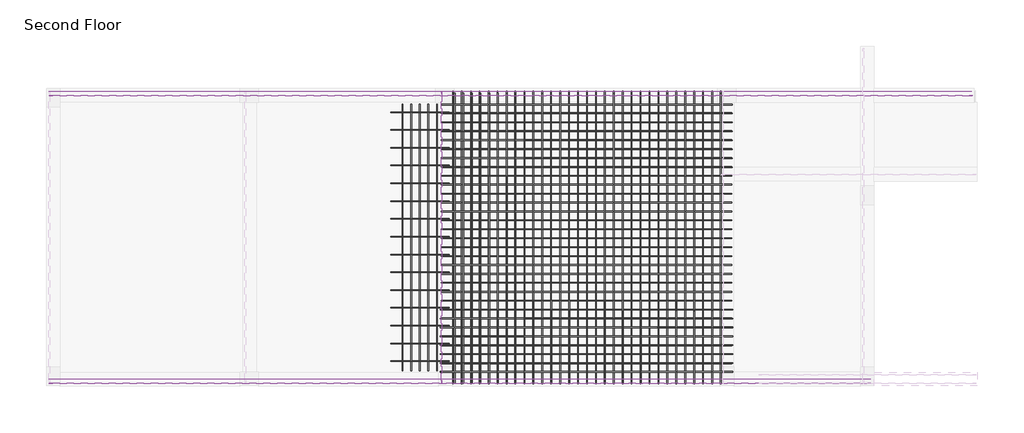
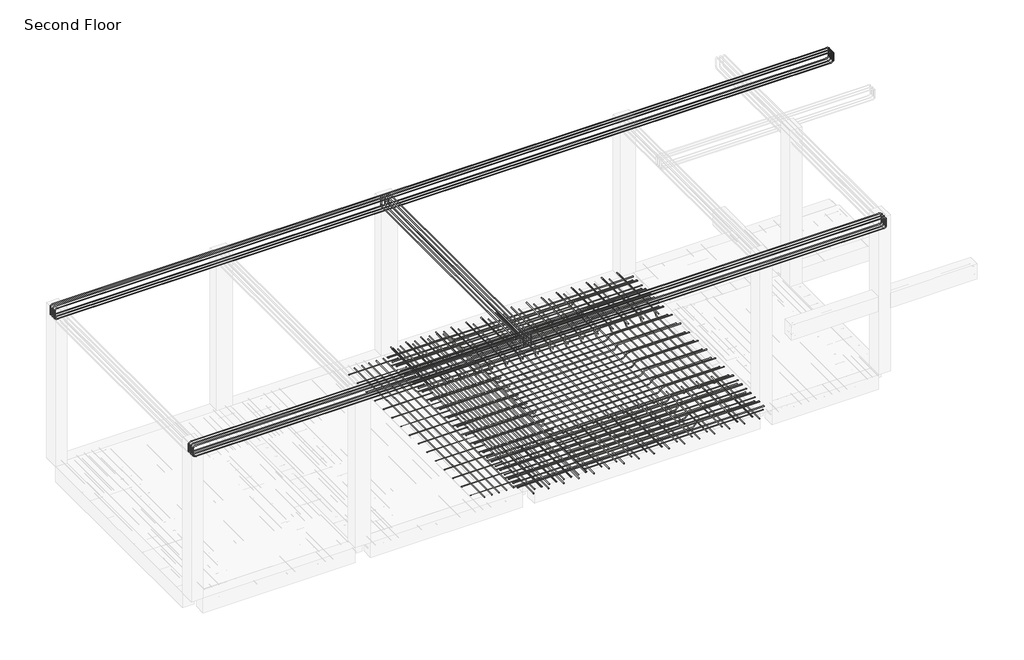
# One storey, part 3 of 4: 18 reinforcing bars.
"""IFC4 building model written with IfcOpenShell, lengths in millimetres."""

from ifc_helpers import new_model, si_unit, point, frame, origin, place, context, project, spatial, polyline, circle_curve, trimmed, segment, composite_curve, source, transform, mapped, element, save
from ifc_brep_helpers import swept_disk

model = new_model("IFC4")

# Units and contexts
model_context = context("Model", 3, world=origin())
ifc_project = project(units=[si_unit("LENGTHUNIT", "METRE", prefix="MILLI")], contexts=[model_context])

# Site, building, storey
site = spatial("IfcSite", under=ifc_project)
building = spatial("IfcBuilding", under=site)
storey = spatial("IfcBuildingStorey", under=building, Name="Second Floor", Elevation=6400.8)

# Reinforcing bars
placement = place(None, origin())
reinforcing_bar_shape = source(origin(), model_context, "Body", "SolidModel", [
    swept_disk(composite_curve([segment(polyline([(-2909.6112474, 5017.2334631, 9364.0994949), (-2909.6112474, 5017.2334631, 9512.0994949)]), True, "CONTINUOUS"), segment(trimmed(circle_curve(frame((-2909.6112474, 4971.2334631, 9512.0994949), z_axis=(1.0, 0.0, 0.0), x_axis=(0.0, 46.0, 0.0)), 46.0), [point((-2909.6112474, 5017.2334631, 9512.0994949))], [point((-2909.6112474, 4971.2334631, 9558.0994949))], True, "CARTESIAN"), True, "CONTINUOUS"), segment(polyline([(-2909.6112474, 4971.2334631, 9558.0994949), (-2909.6112474, 278.4334631, 9558.0994949)]), True, "CONTINUOUS"), segment(trimmed(circle_curve(frame((-2909.6112474, 278.4334631, 9512.0994949), z_axis=(1.0, 0.0, 0.0), x_axis=(0.0, 0.0, 46.0)), 46.0), [point((-2909.6112474, 278.4334631, 9558.0994949))], [point((-2909.6112474, 232.4334631, 9512.0994949))], True, "CARTESIAN"), True, "CONTINUOUS"), segment(polyline([(-2909.6112474, 232.4334631, 9512.0994949), (-2909.6112474, 232.4334631, 9364.0994949)]), True, "CONTINUOUS")], self_intersect=False), 6.0),
])
element("IfcReinforcingBar", 1, at=placement, inside=storey, context=model_context, shape_type="MappedRepresentation", body=[
    mapped(reinforcing_bar_shape, transform((0.0, 0.0, 0.0), x_axis=(1.0, 0.0, 0.0), y_axis=(0.0, 1.0, 0.0), z_axis=(0.0, 0.0, 1.0))),
    mapped(reinforcing_bar_shape, transform((71.1994949, 0.0, 0.0), x_axis=(1.0, 0.0, 0.0), y_axis=(0.0, 1.0, 0.0), z_axis=(0.0, 0.0, 1.0))),
    mapped(reinforcing_bar_shape, transform((142.3989899, 0.0, 0.0), x_axis=(1.0, 0.0, 0.0), y_axis=(0.0, 1.0, 0.0), z_axis=(0.0, 0.0, 1.0))),
])
reinforcing_bar_2_shape = source(origin(), model_context, "Body", "SolidModel", [
    swept_disk(composite_curve([segment(polyline([(-2909.6112474, 5017.2334631, 9533.5005051), (-2909.6112474, 5017.2334631, 9385.5005051)]), True, "CONTINUOUS"), segment(trimmed(circle_curve(frame((-2909.6112474, 4971.2334631, 9385.5005051), z_axis=(-1.0, 0.0, 0.0), x_axis=(0.0, 46.0, 0.0)), 46.0), [point((-2909.6112474, 5017.2334631, 9385.5005051))], [point((-2909.6112474, 4971.2334631, 9339.5005051))], True, "CARTESIAN"), True, "CONTINUOUS"), segment(polyline([(-2909.6112474, 4971.2334631, 9339.5005051), (-2909.6112474, 278.4334631, 9339.5005051)]), True, "CONTINUOUS"), segment(trimmed(circle_curve(frame((-2909.6112474, 278.4334631, 9385.5005051), z_axis=(-1.0, 0.0, 0.0), x_axis=(0.0, 0.0, -46.0)), 46.0), [point((-2909.6112474, 278.4334631, 9339.5005051))], [point((-2909.6112474, 232.4334631, 9385.5005051))], True, "CARTESIAN"), True, "CONTINUOUS"), segment(polyline([(-2909.6112474, 232.4334631, 9385.5005051), (-2909.6112474, 232.4334631, 9533.5005051)]), True, "CONTINUOUS")], self_intersect=False), 6.0),
])
element("IfcReinforcingBar", 2, at=placement, inside=storey, context=model_context, shape_type="MappedRepresentation", body=[
    mapped(reinforcing_bar_2_shape, transform((0.0, 0.0, 0.0), x_axis=(1.0, 0.0, 0.0), y_axis=(0.0, 1.0, 0.0), z_axis=(0.0, 0.0, 1.0))),
    mapped(reinforcing_bar_2_shape, transform((71.1994949, 0.0, 0.0), x_axis=(1.0, 0.0, 0.0), y_axis=(0.0, 1.0, 0.0), z_axis=(0.0, 0.0, 1.0))),
    mapped(reinforcing_bar_2_shape, transform((142.3989899, 0.0, 0.0), x_axis=(1.0, 0.0, 0.0), y_axis=(0.0, 1.0, 0.0), z_axis=(0.0, 0.0, 1.0))),
])
reinforcing_bar_3_shape = source(origin(), model_context, "Body", "SolidModel", [
    swept_disk(composite_curve([segment(polyline([(-9325.7296265, 229.5339681, 9364.0994949), (-9325.7296265, 229.5339681, 9512.0994949)]), True, "CONTINUOUS"), segment(trimmed(circle_curve(frame((-9279.7296265, 229.5339681, 9512.0994949), z_axis=(0.0, 1.0, 0.0), x_axis=(-46.0, 0.0, 0.0)), 46.0), [point((-9325.7296265, 229.5339681, 9512.0994949))], [point((-9279.7296265, 229.5339681, 9558.0994949))], True, "CARTESIAN"), True, "CONTINUOUS"), segment(polyline([(-9279.7296265, 229.5339681, 9558.0994949), (4070.8650323, 229.5339681, 9558.0994949)]), True, "CONTINUOUS"), segment(trimmed(circle_curve(frame((4070.8650323, 229.5339681, 9512.0994949), z_axis=(0.0, 1.0, 0.0), x_axis=(0.0, 0.0, 46.0)), 46.0), [point((4070.8650323, 229.5339681, 9558.0994949))], [point((4116.8650323, 229.5339681, 9512.0994949))], True, "CARTESIAN"), True, "CONTINUOUS"), segment(polyline([(4116.8650323, 229.5339681, 9512.0994949), (4116.8650323, 229.5339681, 9364.0994949)]), True, "CONTINUOUS")], self_intersect=False), 6.0),
])
element("IfcReinforcingBar", 3, at=placement, inside=storey, context=model_context, shape_type="MappedRepresentation", body=[
    mapped(reinforcing_bar_3_shape, transform((0.0, 0.0, 0.0), x_axis=(1.0, 0.0, 0.0), y_axis=(0.0, 1.0, 0.0), z_axis=(0.0, 0.0, 1.0))),
    mapped(reinforcing_bar_3_shape, transform((0.0, 71.1994949, 0.0), x_axis=(1.0, 0.0, 0.0), y_axis=(0.0, 1.0, 0.0), z_axis=(0.0, 0.0, 1.0))),
    mapped(reinforcing_bar_3_shape, transform((0.0, 142.3989899, 0.0), x_axis=(1.0, 0.0, 0.0), y_axis=(0.0, 1.0, 0.0), z_axis=(0.0, 0.0, 1.0))),
])
reinforcing_bar_4_shape = source(origin(), model_context, "Body", "SolidModel", [
    swept_disk(composite_curve([segment(polyline([(-9326.1203644, 229.5339681, 9533.5005051), (-9326.1203644, 229.5339681, 9385.5005051)]), True, "CONTINUOUS"), segment(trimmed(circle_curve(frame((-9280.1203644, 229.5339681, 9385.5005051), z_axis=(0.0, -1.0, 0.0), x_axis=(-46.0, 0.0, 0.0)), 46.0), [point((-9326.1203644, 229.5339681, 9385.5005051))], [point((-9280.1203644, 229.5339681, 9339.5005051))], True, "CARTESIAN"), True, "CONTINUOUS"), segment(polyline([(-9280.1203644, 229.5339681, 9339.5005051), (4076.5679264, 229.5339681, 9339.5005051)]), True, "CONTINUOUS"), segment(trimmed(circle_curve(frame((4076.5679264, 229.5339681, 9385.5005051), z_axis=(0.0, -1.0, 0.0), x_axis=(0.0, 0.0, -46.0)), 46.0), [point((4076.5679264, 229.5339681, 9339.5005051))], [point((4122.5679264, 229.5339681, 9385.5005051))], True, "CARTESIAN"), True, "CONTINUOUS"), segment(polyline([(4122.5679264, 229.5339681, 9385.5005051), (4122.5679264, 229.5339681, 9533.5005051)]), True, "CONTINUOUS")], self_intersect=False), 6.0),
])
element("IfcReinforcingBar", 4, at=placement, inside=storey, context=model_context, shape_type="MappedRepresentation", body=[
    mapped(reinforcing_bar_4_shape, transform((0.0, 0.0, 0.0), x_axis=(1.0, 0.0, 0.0), y_axis=(0.0, 1.0, 0.0), z_axis=(0.0, 0.0, 1.0))),
    mapped(reinforcing_bar_4_shape, transform((0.0, 71.1994949, 0.0), x_axis=(1.0, 0.0, 0.0), y_axis=(0.0, 1.0, 0.0), z_axis=(0.0, 0.0, 1.0))),
    mapped(reinforcing_bar_4_shape, transform((0.0, 142.3989899, 0.0), x_axis=(1.0, 0.0, 0.0), y_axis=(0.0, 1.0, 0.0), z_axis=(0.0, 0.0, 1.0))),
])
reinforcing_bar_5_shape = source(origin(), model_context, "Body", "SolidModel", [
    swept_disk(composite_curve([segment(polyline([(-9325.7296265, 4877.7339681, 9364.0994949), (-9325.7296265, 4877.7339681, 9512.0994949)]), True, "CONTINUOUS"), segment(trimmed(circle_curve(frame((-9279.7296265, 4877.7339681, 9512.0994949), z_axis=(0.0, 1.0, 0.0), x_axis=(-46.0, 0.0, 0.0)), 46.0), [point((-9325.7296265, 4877.7339681, 9512.0994949))], [point((-9279.7296265, 4877.7339681, 9558.0994949))], True, "CARTESIAN"), True, "CONTINUOUS"), segment(polyline([(-9279.7296265, 4877.7339681, 9558.0994949), (5739.4882476, 4877.7339681, 9558.0994949)]), True, "CONTINUOUS"), segment(trimmed(circle_curve(frame((5739.4882476, 4877.7339681, 9512.0994949), z_axis=(0.0, 1.0, 0.0), x_axis=(0.0, 0.0, 46.0)), 46.0), [point((5739.4882476, 4877.7339681, 9558.0994949))], [point((5785.4882476, 4877.7339681, 9512.0994949))], True, "CARTESIAN"), True, "CONTINUOUS"), segment(polyline([(5785.4882476, 4877.7339681, 9512.0994949), (5785.4882476, 4877.7339681, 9364.0994949)]), True, "CONTINUOUS")], self_intersect=False), 6.0),
])
element("IfcReinforcingBar", 5, at=placement, inside=storey, context=model_context, shape_type="MappedRepresentation", body=[
    mapped(reinforcing_bar_5_shape, transform((0.0, 0.0, 0.0), x_axis=(1.0, 0.0, 0.0), y_axis=(0.0, 1.0, 0.0), z_axis=(0.0, 0.0, 1.0))),
    mapped(reinforcing_bar_5_shape, transform((0.0, 71.1994949, 0.0), x_axis=(1.0, 0.0, 0.0), y_axis=(0.0, 1.0, 0.0), z_axis=(0.0, 0.0, 1.0))),
    mapped(reinforcing_bar_5_shape, transform((0.0, 142.3989899, 0.0), x_axis=(1.0, 0.0, 0.0), y_axis=(0.0, 1.0, 0.0), z_axis=(0.0, 0.0, 1.0))),
])
reinforcing_bar_6_shape = source(origin(), model_context, "Body", "SolidModel", [
    swept_disk(composite_curve([segment(polyline([(-9326.1203644, 4877.7339681, 9533.5005051), (-9326.1203644, 4877.7339681, 9385.5005051)]), True, "CONTINUOUS"), segment(trimmed(circle_curve(frame((-9280.1203644, 4877.7339681, 9385.5005051), z_axis=(0.0, -1.0, 0.0), x_axis=(-46.0, 0.0, 0.0)), 46.0), [point((-9326.1203644, 4877.7339681, 9385.5005051))], [point((-9280.1203644, 4877.7339681, 9339.5005051))], True, "CARTESIAN"), True, "CONTINUOUS"), segment(polyline([(-9280.1203644, 4877.7339681, 9339.5005051), (5727.8951301, 4877.7339681, 9339.5005051)]), True, "CONTINUOUS"), segment(trimmed(circle_curve(frame((5727.8951301, 4877.7339681, 9385.5005051), z_axis=(0.0, -1.0, 0.0), x_axis=(0.0, 0.0, -46.0)), 46.0), [point((5727.8951301, 4877.7339681, 9339.5005051))], [point((5773.8951301, 4877.7339681, 9385.5005051))], True, "CARTESIAN"), True, "CONTINUOUS"), segment(polyline([(5773.8951301, 4877.7339681, 9385.5005051), (5773.8951301, 4877.7339681, 9533.5005051)]), True, "CONTINUOUS")], self_intersect=False), 6.0),
])
element("IfcReinforcingBar", 6, at=placement, inside=storey, context=model_context, shape_type="MappedRepresentation", body=[
    mapped(reinforcing_bar_6_shape, transform((0.0, 0.0, 0.0), x_axis=(1.0, 0.0, 0.0), y_axis=(0.0, 1.0, 0.0), z_axis=(0.0, 0.0, 1.0))),
    mapped(reinforcing_bar_6_shape, transform((0.0, 71.1994949, 0.0), x_axis=(1.0, 0.0, 0.0), y_axis=(0.0, 1.0, 0.0), z_axis=(0.0, 0.0, 1.0))),
    mapped(reinforcing_bar_6_shape, transform((0.0, 142.3989899, 0.0), x_axis=(1.0, 0.0, 0.0), y_axis=(0.0, 1.0, 0.0), z_axis=(0.0, 0.0, 1.0))),
])
reinforcing_bar_7_shape = source(origin(), model_context, "Body", "SolidModel", [
    swept_disk(composite_curve([segment(polyline([(-3546.4250876, 4809.6334631, 6359.5006995), (-3546.4250876, 440.0334631, 6359.5006995)]), True, "CONTINUOUS")], self_intersect=False), 6.0),
])
element("IfcReinforcingBar", 7, at=placement, inside=storey, context=model_context, shape_type="MappedRepresentation", body=[
    mapped(reinforcing_bar_7_shape, transform((0.0, 0.0, 0.0), x_axis=(1.0, 0.0, 0.0), y_axis=(0.0, 1.0, 0.0), z_axis=(0.0, 0.0, 1.0))),
    mapped(reinforcing_bar_7_shape, transform((140.6783338, 0.0, 0.0), x_axis=(1.0, 0.0, 0.0), y_axis=(0.0, 1.0, 0.0), z_axis=(0.0, 0.0, 1.0))),
    mapped(reinforcing_bar_7_shape, transform((281.3566676, 0.0, 0.0), x_axis=(1.0, 0.0, 0.0), y_axis=(0.0, 1.0, 0.0), z_axis=(0.0, 0.0, 1.0))),
    mapped(reinforcing_bar_7_shape, transform((422.0350014, 0.0, 0.0), x_axis=(1.0, 0.0, 0.0), y_axis=(0.0, 1.0, 0.0), z_axis=(0.0, 0.0, 1.0))),
    mapped(reinforcing_bar_7_shape, transform((562.7133352, 0.0, 0.0), x_axis=(1.0, 0.0, 0.0), y_axis=(0.0, 1.0, 0.0), z_axis=(0.0, 0.0, 1.0))),
])
reinforcing_bar_8_shape = source(origin(), model_context, "Body", "SolidModel", [
    swept_disk(composite_curve([segment(polyline([(-2778.2123639, 4678.4115375, 6371.8), (-3737.2865297, 4678.4115375, 6371.8)]), True, "CONTINUOUS")], self_intersect=False), 4.0),
])
element("IfcReinforcingBar", 8, at=placement, inside=storey, context=model_context, shape_type="MappedRepresentation", body=[
    mapped(reinforcing_bar_8_shape, transform((0.0, 0.0, 0.0), x_axis=(1.0, 0.0, 0.0), y_axis=(0.0, 1.0, 0.0), z_axis=(0.0, 0.0, 1.0))),
    mapped(reinforcing_bar_8_shape, transform((0.0, -291.8025106, 0.0), x_axis=(1.0, 0.0, 0.0), y_axis=(0.0, 1.0, 0.0), z_axis=(0.0, 0.0, 1.0))),
    mapped(reinforcing_bar_8_shape, transform((0.0, -583.6050212, 0.0), x_axis=(1.0, 0.0, 0.0), y_axis=(0.0, 1.0, 0.0), z_axis=(0.0, 0.0, 1.0))),
    mapped(reinforcing_bar_8_shape, transform((0.0, -875.4075319, 0.0), x_axis=(1.0, 0.0, 0.0), y_axis=(0.0, 1.0, 0.0), z_axis=(0.0, 0.0, 1.0))),
    mapped(reinforcing_bar_8_shape, transform((0.0, -1167.2100425, 0.0), x_axis=(1.0, 0.0, 0.0), y_axis=(0.0, 1.0, 0.0), z_axis=(0.0, 0.0, 1.0))),
    mapped(reinforcing_bar_8_shape, transform((0.0, -1459.0125531, 0.0), x_axis=(1.0, 0.0, 0.0), y_axis=(0.0, 1.0, 0.0), z_axis=(0.0, 0.0, 1.0))),
    mapped(reinforcing_bar_8_shape, transform((0.0, -1750.8150637, 0.0), x_axis=(1.0, 0.0, 0.0), y_axis=(0.0, 1.0, 0.0), z_axis=(0.0, 0.0, 1.0))),
    mapped(reinforcing_bar_8_shape, transform((0.0, -2042.6175743, 0.0), x_axis=(1.0, 0.0, 0.0), y_axis=(0.0, 1.0, 0.0), z_axis=(0.0, 0.0, 1.0))),
    mapped(reinforcing_bar_8_shape, transform((0.0, -2334.420085, 0.0), x_axis=(1.0, 0.0, 0.0), y_axis=(0.0, 1.0, 0.0), z_axis=(0.0, 0.0, 1.0))),
    mapped(reinforcing_bar_8_shape, transform((0.0, -2626.2225956, 0.0), x_axis=(1.0, 0.0, 0.0), y_axis=(0.0, 1.0, 0.0), z_axis=(0.0, 0.0, 1.0))),
    mapped(reinforcing_bar_8_shape, transform((0.0, -2918.0251062, 0.0), x_axis=(1.0, 0.0, 0.0), y_axis=(0.0, 1.0, 0.0), z_axis=(0.0, 0.0, 1.0))),
    mapped(reinforcing_bar_8_shape, transform((0.0, -3209.8276168, 0.0), x_axis=(1.0, 0.0, 0.0), y_axis=(0.0, 1.0, 0.0), z_axis=(0.0, 0.0, 1.0))),
    mapped(reinforcing_bar_8_shape, transform((0.0, -3501.6301274, 0.0), x_axis=(1.0, 0.0, 0.0), y_axis=(0.0, 1.0, 0.0), z_axis=(0.0, 0.0, 1.0))),
    mapped(reinforcing_bar_8_shape, transform((0.0, -3793.4326381, 0.0), x_axis=(1.0, 0.0, 0.0), y_axis=(0.0, 1.0, 0.0), z_axis=(0.0, 0.0, 1.0))),
    mapped(reinforcing_bar_8_shape, transform((0.0, -4085.2351487, 0.0), x_axis=(1.0, 0.0, 0.0), y_axis=(0.0, 1.0, 0.0), z_axis=(0.0, 0.0, 1.0))),
])
reinforcing_bar_9_shape = source(origin(), model_context, "Body", "SolidModel", [
    swept_disk(composite_curve([segment(polyline([(-1702.6950858, 4992.3164819, 6354.5006995), (-1702.6950858, 234.3272052, 6354.5006995)]), True, "CONTINUOUS")], self_intersect=False), 6.0),
])
element("IfcReinforcingBar", 9, at=placement, inside=storey, context=model_context, shape_type="MappedRepresentation", body=[
    mapped(reinforcing_bar_9_shape, transform((0.0, 0.0, 0.0), x_axis=(1.0, 0.0, 0.0), y_axis=(0.0, 1.0, 0.0), z_axis=(0.0, 0.0, 1.0))),
    mapped(reinforcing_bar_9_shape, transform((-141.4880952, 0.0, 0.0), x_axis=(1.0, 0.0, 0.0), y_axis=(0.0, 1.0, 0.0), z_axis=(0.0, 0.0, 1.0))),
    mapped(reinforcing_bar_9_shape, transform((-282.9761905, 0.0, 0.0), x_axis=(1.0, 0.0, 0.0), y_axis=(0.0, 1.0, 0.0), z_axis=(0.0, 0.0, 1.0))),
    mapped(reinforcing_bar_9_shape, transform((-424.4642857, 0.0, 0.0), x_axis=(1.0, 0.0, 0.0), y_axis=(0.0, 1.0, 0.0), z_axis=(0.0, 0.0, 1.0))),
    mapped(reinforcing_bar_9_shape, transform((-565.952381, 0.0, 0.0), x_axis=(1.0, 0.0, 0.0), y_axis=(0.0, 1.0, 0.0), z_axis=(0.0, 0.0, 1.0))),
    mapped(reinforcing_bar_9_shape, transform((-707.4404762, 0.0, 0.0), x_axis=(1.0, 0.0, 0.0), y_axis=(0.0, 1.0, 0.0), z_axis=(0.0, 0.0, 1.0))),
    mapped(reinforcing_bar_9_shape, transform((-848.9285714, 0.0, 0.0), x_axis=(1.0, 0.0, 0.0), y_axis=(0.0, 1.0, 0.0), z_axis=(0.0, 0.0, 1.0))),
    mapped(reinforcing_bar_9_shape, transform((-990.4166667, 0.0, 0.0), x_axis=(1.0, 0.0, 0.0), y_axis=(0.0, 1.0, 0.0), z_axis=(0.0, 0.0, 1.0))),
])
reinforcing_bar_10_shape = source(origin(), model_context, "Body", "SolidModel", [
    swept_disk(composite_curve([segment(polyline([(-2905.905155, 4803.6334631, 6366.7687876), (-1727.9771661, 4803.6334631, 6366.7687876)]), True, "CONTINUOUS"), segment(trimmed(circle_curve(frame((-1727.9771661, 4803.6334631, 6320.7687876), z_axis=(0.0, 1.0, 0.0), x_axis=(0.0, 0.0, 46.0)), 46.0), [point((-1727.9771661, 4803.6334631, 6366.7687876))], [point((-1695.4502541, 4803.6334631, 6353.2956996))], True, "CARTESIAN"), True, "CONTINUOUS"), segment(polyline([(-1695.4502541, 4803.6334631, 6353.2956996), (-1634.9899166, 4803.6334631, 6292.8353621)]), True, "CONTINUOUS"), segment(trimmed(circle_curve(frame((-1602.4630047, 4803.6334631, 6325.362274), z_axis=(0.0, -1.0, 0.0), x_axis=(-32.52691189999996, 0.0, -32.526911900000414)), 46.0), [point((-1634.9899166, 4803.6334631, 6292.8353621))], [point((-1602.4630047, 4803.6334631, 6279.362274))], True, "CARTESIAN"), True, "CONTINUOUS"), segment(polyline([(-1602.4630047, 4803.6334631, 6279.362274), (1847.5013288, 4803.6334631, 6279.362274)]), True, "CONTINUOUS")], self_intersect=False), 6.0),
])
element("IfcReinforcingBar", 10, at=placement, inside=storey, context=model_context, shape_type="MappedRepresentation", body=[
    mapped(reinforcing_bar_10_shape, transform((0.0, 0.0, 0.0), x_axis=(1.0, 0.0, 0.0), y_axis=(0.0, 1.0, 0.0), z_axis=(0.0, 0.0, 1.0))),
    mapped(reinforcing_bar_10_shape, transform((0.0, -292.3066667, 0.0), x_axis=(1.0, 0.0, 0.0), y_axis=(0.0, 1.0, 0.0), z_axis=(0.0, 0.0, 1.0))),
    mapped(reinforcing_bar_10_shape, transform((0.0, -584.6133333, 0.0), x_axis=(1.0, 0.0, 0.0), y_axis=(0.0, 1.0, 0.0), z_axis=(0.0, 0.0, 1.0))),
    mapped(reinforcing_bar_10_shape, transform((0.0, -876.92, 0.0), x_axis=(1.0, 0.0, 0.0), y_axis=(0.0, 1.0, 0.0), z_axis=(0.0, 0.0, 1.0))),
    mapped(reinforcing_bar_10_shape, transform((0.0, -1169.2266667, 0.0), x_axis=(1.0, 0.0, 0.0), y_axis=(0.0, 1.0, 0.0), z_axis=(0.0, 0.0, 1.0))),
    mapped(reinforcing_bar_10_shape, transform((0.0, -1461.5333333, 0.0), x_axis=(1.0, 0.0, 0.0), y_axis=(0.0, 1.0, 0.0), z_axis=(0.0, 0.0, 1.0))),
    mapped(reinforcing_bar_10_shape, transform((0.0, -1753.84, 0.0), x_axis=(1.0, 0.0, 0.0), y_axis=(0.0, 1.0, 0.0), z_axis=(0.0, 0.0, 1.0))),
    mapped(reinforcing_bar_10_shape, transform((0.0, -2046.1466667, 0.0), x_axis=(1.0, 0.0, 0.0), y_axis=(0.0, 1.0, 0.0), z_axis=(0.0, 0.0, 1.0))),
    mapped(reinforcing_bar_10_shape, transform((0.0, -2338.4533333, 0.0), x_axis=(1.0, 0.0, 0.0), y_axis=(0.0, 1.0, 0.0), z_axis=(0.0, 0.0, 1.0))),
    mapped(reinforcing_bar_10_shape, transform((0.0, -2630.76, 0.0), x_axis=(1.0, 0.0, 0.0), y_axis=(0.0, 1.0, 0.0), z_axis=(0.0, 0.0, 1.0))),
    mapped(reinforcing_bar_10_shape, transform((0.0, -2923.0666667, 0.0), x_axis=(1.0, 0.0, 0.0), y_axis=(0.0, 1.0, 0.0), z_axis=(0.0, 0.0, 1.0))),
    mapped(reinforcing_bar_10_shape, transform((0.0, -3215.3733333, 0.0), x_axis=(1.0, 0.0, 0.0), y_axis=(0.0, 1.0, 0.0), z_axis=(0.0, 0.0, 1.0))),
    mapped(reinforcing_bar_10_shape, transform((0.0, -3507.68, 0.0), x_axis=(1.0, 0.0, 0.0), y_axis=(0.0, 1.0, 0.0), z_axis=(0.0, 0.0, 1.0))),
    mapped(reinforcing_bar_10_shape, transform((0.0, -3799.9866667, 0.0), x_axis=(1.0, 0.0, 0.0), y_axis=(0.0, 1.0, 0.0), z_axis=(0.0, 0.0, 1.0))),
    mapped(reinforcing_bar_10_shape, transform((0.0, -4092.2933333, 0.0), x_axis=(1.0, 0.0, 0.0), y_axis=(0.0, 1.0, 0.0), z_axis=(0.0, 0.0, 1.0))),
    mapped(reinforcing_bar_10_shape, transform((0.0, -4384.6, 0.0), x_axis=(1.0, 0.0, 0.0), y_axis=(0.0, 1.0, 0.0), z_axis=(0.0, 0.0, 1.0))),
])
reinforcing_bar_11_shape = source(origin(), model_context, "Body", "SolidModel", [
    swept_disk(composite_curve([segment(polyline([(-2911.6309684, 4803.6334631, 6364.2017937), (-1557.9199073, 4803.6334631, 6364.2017937)]), True, "CONTINUOUS")], self_intersect=False), 6.0),
])
element("IfcReinforcingBar", 11, at=placement, inside=storey, context=model_context, shape_type="MappedRepresentation", body=[
    mapped(reinforcing_bar_11_shape, transform((0.0, 0.0, 0.0), x_axis=(1.0, 0.0, 0.0), y_axis=(0.0, 1.0, 0.0), z_axis=(0.0, 0.0, 1.0))),
    mapped(reinforcing_bar_11_shape, transform((0.0, -292.3066667, 0.0), x_axis=(1.0, 0.0, 0.0), y_axis=(0.0, 1.0, 0.0), z_axis=(0.0, 0.0, 1.0))),
    mapped(reinforcing_bar_11_shape, transform((0.0, -584.6133333, 0.0), x_axis=(1.0, 0.0, 0.0), y_axis=(0.0, 1.0, 0.0), z_axis=(0.0, 0.0, 1.0))),
    mapped(reinforcing_bar_11_shape, transform((0.0, -876.92, 0.0), x_axis=(1.0, 0.0, 0.0), y_axis=(0.0, 1.0, 0.0), z_axis=(0.0, 0.0, 1.0))),
    mapped(reinforcing_bar_11_shape, transform((0.0, -1169.2266667, 0.0), x_axis=(1.0, 0.0, 0.0), y_axis=(0.0, 1.0, 0.0), z_axis=(0.0, 0.0, 1.0))),
    mapped(reinforcing_bar_11_shape, transform((0.0, -1461.5333333, 0.0), x_axis=(1.0, 0.0, 0.0), y_axis=(0.0, 1.0, 0.0), z_axis=(0.0, 0.0, 1.0))),
    mapped(reinforcing_bar_11_shape, transform((0.0, -1753.84, 0.0), x_axis=(1.0, 0.0, 0.0), y_axis=(0.0, 1.0, 0.0), z_axis=(0.0, 0.0, 1.0))),
    mapped(reinforcing_bar_11_shape, transform((0.0, -2046.1466667, 0.0), x_axis=(1.0, 0.0, 0.0), y_axis=(0.0, 1.0, 0.0), z_axis=(0.0, 0.0, 1.0))),
    mapped(reinforcing_bar_11_shape, transform((0.0, -2338.4533333, 0.0), x_axis=(1.0, 0.0, 0.0), y_axis=(0.0, 1.0, 0.0), z_axis=(0.0, 0.0, 1.0))),
    mapped(reinforcing_bar_11_shape, transform((0.0, -2630.76, 0.0), x_axis=(1.0, 0.0, 0.0), y_axis=(0.0, 1.0, 0.0), z_axis=(0.0, 0.0, 1.0))),
    mapped(reinforcing_bar_11_shape, transform((0.0, -2923.0666667, 0.0), x_axis=(1.0, 0.0, 0.0), y_axis=(0.0, 1.0, 0.0), z_axis=(0.0, 0.0, 1.0))),
    mapped(reinforcing_bar_11_shape, transform((0.0, -3215.3733333, 0.0), x_axis=(1.0, 0.0, 0.0), y_axis=(0.0, 1.0, 0.0), z_axis=(0.0, 0.0, 1.0))),
    mapped(reinforcing_bar_11_shape, transform((0.0, -3507.68, 0.0), x_axis=(1.0, 0.0, 0.0), y_axis=(0.0, 1.0, 0.0), z_axis=(0.0, 0.0, 1.0))),
    mapped(reinforcing_bar_11_shape, transform((0.0, -3799.9866667, 0.0), x_axis=(1.0, 0.0, 0.0), y_axis=(0.0, 1.0, 0.0), z_axis=(0.0, 0.0, 1.0))),
    mapped(reinforcing_bar_11_shape, transform((0.0, -4092.2933333, 0.0), x_axis=(1.0, 0.0, 0.0), y_axis=(0.0, 1.0, 0.0), z_axis=(0.0, 0.0, 1.0))),
    mapped(reinforcing_bar_11_shape, transform((0.0, -4384.6, 0.0), x_axis=(1.0, 0.0, 0.0), y_axis=(0.0, 1.0, 0.0), z_axis=(0.0, 0.0, 1.0))),
])
reinforcing_bar_12_shape = source(origin(), model_context, "Body", "SolidModel", [
    swept_disk(composite_curve([segment(polyline([(1849.122149, 559.2793552, 6366.7687876), (670.8521547, 559.2793552, 6366.7687876)]), True, "CONTINUOUS"), segment(trimmed(circle_curve(frame((670.8521547, 559.2793552, 6320.7687876), z_axis=(0.0, -1.0, 0.0), x_axis=(0.0, 0.0, 46.0)), 46.0), [point((670.8521547, 559.2793552, 6366.7687876))], [point((638.3252427, 559.2793552, 6353.2956996))], True, "CARTESIAN"), True, "CONTINUOUS"), segment(polyline([(638.3252427, 559.2793552, 6353.2956996), (577.8649052, 559.2793552, 6292.8353621)]), True, "CONTINUOUS"), segment(trimmed(circle_curve(frame((545.3379933, 559.2793552, 6325.362274), z_axis=(0.0, 1.0000000000000002, 0.0), x_axis=(32.52691189999996, 0.0, -32.526911900000414)), 46.0), [point((577.8649052, 559.2793552, 6292.8353621))], [point((545.3379933, 559.2793552, 6279.362274))], True, "CARTESIAN"), True, "CONTINUOUS"), segment(polyline([(545.3379933, 559.2793552, 6279.362274), (-2914.2248337, 559.2793552, 6279.362274)]), True, "CONTINUOUS")], self_intersect=False), 6.0),
])
element("IfcReinforcingBar", 12, at=placement, inside=storey, context=model_context, shape_type="MappedRepresentation", body=[
    mapped(reinforcing_bar_12_shape, transform((0.0, 0.0, 0.0), x_axis=(1.0, 0.0, 0.0), y_axis=(0.0, 1.0, 0.0), z_axis=(0.0, 0.0, 1.0))),
    mapped(reinforcing_bar_12_shape, transform((0.0, 293.1320516, 0.0), x_axis=(1.0, 0.0, 0.0), y_axis=(0.0, 1.0, 0.0), z_axis=(0.0, 0.0, 1.0))),
    mapped(reinforcing_bar_12_shape, transform((0.0, 586.2641031, 0.0), x_axis=(1.0, 0.0, 0.0), y_axis=(0.0, 1.0, 0.0), z_axis=(0.0, 0.0, 1.0))),
    mapped(reinforcing_bar_12_shape, transform((0.0, 879.3961547, 0.0), x_axis=(1.0, 0.0, 0.0), y_axis=(0.0, 1.0, 0.0), z_axis=(0.0, 0.0, 1.0))),
    mapped(reinforcing_bar_12_shape, transform((0.0, 1172.5282063, 0.0), x_axis=(1.0, 0.0, 0.0), y_axis=(0.0, 1.0, 0.0), z_axis=(0.0, 0.0, 1.0))),
    mapped(reinforcing_bar_12_shape, transform((0.0, 1465.6602578, 0.0), x_axis=(1.0, 0.0, 0.0), y_axis=(0.0, 1.0, 0.0), z_axis=(0.0, 0.0, 1.0))),
    mapped(reinforcing_bar_12_shape, transform((0.0, 1758.7923094, 0.0), x_axis=(1.0, 0.0, 0.0), y_axis=(0.0, 1.0, 0.0), z_axis=(0.0, 0.0, 1.0))),
    mapped(reinforcing_bar_12_shape, transform((0.0, 2051.924361, 0.0), x_axis=(1.0, 0.0, 0.0), y_axis=(0.0, 1.0, 0.0), z_axis=(0.0, 0.0, 1.0))),
    mapped(reinforcing_bar_12_shape, transform((0.0, 2345.0564125, 0.0), x_axis=(1.0, 0.0, 0.0), y_axis=(0.0, 1.0, 0.0), z_axis=(0.0, 0.0, 1.0))),
    mapped(reinforcing_bar_12_shape, transform((0.0, 2638.1884641, 0.0), x_axis=(1.0, 0.0, 0.0), y_axis=(0.0, 1.0, 0.0), z_axis=(0.0, 0.0, 1.0))),
    mapped(reinforcing_bar_12_shape, transform((0.0, 2931.3205157, 0.0), x_axis=(1.0, 0.0, 0.0), y_axis=(0.0, 1.0, 0.0), z_axis=(0.0, 0.0, 1.0))),
    mapped(reinforcing_bar_12_shape, transform((0.0, 3224.4525672, 0.0), x_axis=(1.0, 0.0, 0.0), y_axis=(0.0, 1.0, 0.0), z_axis=(0.0, 0.0, 1.0))),
    mapped(reinforcing_bar_12_shape, transform((0.0, 3517.5846188, 0.0), x_axis=(1.0, 0.0, 0.0), y_axis=(0.0, 1.0, 0.0), z_axis=(0.0, 0.0, 1.0))),
    mapped(reinforcing_bar_12_shape, transform((0.0, 3810.7166704, 0.0), x_axis=(1.0, 0.0, 0.0), y_axis=(0.0, 1.0, 0.0), z_axis=(0.0, 0.0, 1.0))),
    mapped(reinforcing_bar_12_shape, transform((0.0, 4103.848722, 0.0), x_axis=(1.0, 0.0, 0.0), y_axis=(0.0, 1.0, 0.0), z_axis=(0.0, 0.0, 1.0))),
])
reinforcing_bar_13_shape = source(origin(), model_context, "Body", "SolidModel", [
    swept_disk(composite_curve([segment(polyline([(1854.5084921, 3775.4003908, 6354.5006995), (-2903.4807845, 3775.4003908, 6354.5006995)]), True, "CONTINUOUS")], self_intersect=False), 6.0),
])
element("IfcReinforcingBar", 13, at=placement, inside=storey, context=model_context, shape_type="MappedRepresentation", body=[
    mapped(reinforcing_bar_13_shape, transform((0.0, 0.0, 0.0), x_axis=(1.0, 0.0, 0.0), y_axis=(0.0, 1.0, 0.0), z_axis=(0.0, 0.0, 1.0))),
    mapped(reinforcing_bar_13_shape, transform((0.0, 146.8904389, 0.0), x_axis=(1.0, 0.0, 0.0), y_axis=(0.0, 1.0, 0.0), z_axis=(0.0, 0.0, 1.0))),
    mapped(reinforcing_bar_13_shape, transform((0.0, 293.7808778, 0.0), x_axis=(1.0, 0.0, 0.0), y_axis=(0.0, 1.0, 0.0), z_axis=(0.0, 0.0, 1.0))),
    mapped(reinforcing_bar_13_shape, transform((0.0, 440.6713167, 0.0), x_axis=(1.0, 0.0, 0.0), y_axis=(0.0, 1.0, 0.0), z_axis=(0.0, 0.0, 1.0))),
    mapped(reinforcing_bar_13_shape, transform((0.0, 587.5617556, 0.0), x_axis=(1.0, 0.0, 0.0), y_axis=(0.0, 1.0, 0.0), z_axis=(0.0, 0.0, 1.0))),
    mapped(reinforcing_bar_13_shape, transform((0.0, 734.4521945, 0.0), x_axis=(1.0, 0.0, 0.0), y_axis=(0.0, 1.0, 0.0), z_axis=(0.0, 0.0, 1.0))),
    mapped(reinforcing_bar_13_shape, transform((0.0, 881.3426334, 0.0), x_axis=(1.0, 0.0, 0.0), y_axis=(0.0, 1.0, 0.0), z_axis=(0.0, 0.0, 1.0))),
    mapped(reinforcing_bar_13_shape, transform((0.0, 1028.2330723, 0.0), x_axis=(1.0, 0.0, 0.0), y_axis=(0.0, 1.0, 0.0), z_axis=(0.0, 0.0, 1.0))),
])
reinforcing_bar_14_shape = source(origin(), model_context, "Body", "SolidModel", [
    swept_disk(composite_curve([segment(polyline([(1667.8254733, 4978.61046, 6366.7687876), (1667.8254733, 3800.6824711, 6366.7687876)]), True, "CONTINUOUS"), segment(trimmed(circle_curve(frame((1667.8254733, 3800.6824711, 6320.7687876), z_axis=(1.0, 0.0, 0.0), x_axis=(0.0, 0.0, 46.0)), 46.0), [point((1667.8254733, 3800.6824711, 6366.7687876))], [point((1667.8254733, 3768.1555592, 6353.2956996))], True, "CARTESIAN"), True, "CONTINUOUS"), segment(polyline([(1667.8254733, 3768.1555592, 6353.2956996), (1667.8254733, 3707.6952216, 6292.8353621)]), True, "CONTINUOUS"), segment(trimmed(circle_curve(frame((1667.8254733, 3675.1683097, 6325.362274), z_axis=(-1.0, 0.0, 0.0), x_axis=(0.0, 32.52691189999996, -32.526911900000414)), 46.0), [point((1667.8254733, 3707.6952216, 6292.8353621))], [point((1667.8254733, 3675.1683097, 6279.362274))], True, "CARTESIAN"), True, "CONTINUOUS"), segment(polyline([(1667.8254733, 3675.1683097, 6279.362274), (1667.8254733, 225.2039762, 6279.362274)]), True, "CONTINUOUS")], self_intersect=False), 6.0),
])
element("IfcReinforcingBar", 14, at=placement, inside=storey, context=model_context, shape_type="MappedRepresentation", body=[
    mapped(reinforcing_bar_14_shape, transform((0.0, 0.0, 0.0), x_axis=(1.0, 0.0, 0.0), y_axis=(0.0, 1.0, 0.0), z_axis=(0.0, 0.0, 1.0))),
    mapped(reinforcing_bar_14_shape, transform((-292.44, 0.0, 0.0), x_axis=(1.0, 0.0, 0.0), y_axis=(0.0, 1.0, 0.0), z_axis=(0.0, 0.0, 1.0))),
    mapped(reinforcing_bar_14_shape, transform((-584.88, 0.0, 0.0), x_axis=(1.0, 0.0, 0.0), y_axis=(0.0, 1.0, 0.0), z_axis=(0.0, 0.0, 1.0))),
    mapped(reinforcing_bar_14_shape, transform((-877.32, 0.0, 0.0), x_axis=(1.0, 0.0, 0.0), y_axis=(0.0, 1.0, 0.0), z_axis=(0.0, 0.0, 1.0))),
    mapped(reinforcing_bar_14_shape, transform((-1169.76, 0.0, 0.0), x_axis=(1.0, 0.0, 0.0), y_axis=(0.0, 1.0, 0.0), z_axis=(0.0, 0.0, 1.0))),
    mapped(reinforcing_bar_14_shape, transform((-1462.2, 0.0, 0.0), x_axis=(1.0, 0.0, 0.0), y_axis=(0.0, 1.0, 0.0), z_axis=(0.0, 0.0, 1.0))),
    mapped(reinforcing_bar_14_shape, transform((-1754.64, 0.0, 0.0), x_axis=(1.0, 0.0, 0.0), y_axis=(0.0, 1.0, 0.0), z_axis=(0.0, 0.0, 1.0))),
    mapped(reinforcing_bar_14_shape, transform((-2047.08, 0.0, 0.0), x_axis=(1.0, 0.0, 0.0), y_axis=(0.0, 1.0, 0.0), z_axis=(0.0, 0.0, 1.0))),
    mapped(reinforcing_bar_14_shape, transform((-2339.52, 0.0, 0.0), x_axis=(1.0, 0.0, 0.0), y_axis=(0.0, 1.0, 0.0), z_axis=(0.0, 0.0, 1.0))),
    mapped(reinforcing_bar_14_shape, transform((-2631.96, 0.0, 0.0), x_axis=(1.0, 0.0, 0.0), y_axis=(0.0, 1.0, 0.0), z_axis=(0.0, 0.0, 1.0))),
    mapped(reinforcing_bar_14_shape, transform((-2924.4, 0.0, 0.0), x_axis=(1.0, 0.0, 0.0), y_axis=(0.0, 1.0, 0.0), z_axis=(0.0, 0.0, 1.0))),
    mapped(reinforcing_bar_14_shape, transform((-3216.84, 0.0, 0.0), x_axis=(1.0, 0.0, 0.0), y_axis=(0.0, 1.0, 0.0), z_axis=(0.0, 0.0, 1.0))),
    mapped(reinforcing_bar_14_shape, transform((-3509.28, 0.0, 0.0), x_axis=(1.0, 0.0, 0.0), y_axis=(0.0, 1.0, 0.0), z_axis=(0.0, 0.0, 1.0))),
    mapped(reinforcing_bar_14_shape, transform((-3801.72, 0.0, 0.0), x_axis=(1.0, 0.0, 0.0), y_axis=(0.0, 1.0, 0.0), z_axis=(0.0, 0.0, 1.0))),
    mapped(reinforcing_bar_14_shape, transform((-4094.16, 0.0, 0.0), x_axis=(1.0, 0.0, 0.0), y_axis=(0.0, 1.0, 0.0), z_axis=(0.0, 0.0, 1.0))),
    mapped(reinforcing_bar_14_shape, transform((-4386.6, 0.0, 0.0), x_axis=(1.0, 0.0, 0.0), y_axis=(0.0, 1.0, 0.0), z_axis=(0.0, 0.0, 1.0))),
])
reinforcing_bar_15_shape = source(origin(), model_context, "Body", "SolidModel", [
    swept_disk(composite_curve([segment(polyline([(1667.8254733, 5026.3578219, 6364.2017937), (1667.8254733, 3630.6252123, 6364.2017937)]), True, "CONTINUOUS")], self_intersect=False), 6.0),
])
element("IfcReinforcingBar", 15, at=placement, inside=storey, context=model_context, shape_type="MappedRepresentation", body=[
    mapped(reinforcing_bar_15_shape, transform((0.0, 0.0, 0.0), x_axis=(1.0, 0.0, 0.0), y_axis=(0.0, 1.0, 0.0), z_axis=(0.0, 0.0, 1.0))),
    mapped(reinforcing_bar_15_shape, transform((-292.44, 0.0, 0.0), x_axis=(1.0, 0.0, 0.0), y_axis=(0.0, 1.0, 0.0), z_axis=(0.0, 0.0, 1.0))),
    mapped(reinforcing_bar_15_shape, transform((-584.88, 0.0, 0.0), x_axis=(1.0, 0.0, 0.0), y_axis=(0.0, 1.0, 0.0), z_axis=(0.0, 0.0, 1.0))),
    mapped(reinforcing_bar_15_shape, transform((-877.32, 0.0, 0.0), x_axis=(1.0, 0.0, 0.0), y_axis=(0.0, 1.0, 0.0), z_axis=(0.0, 0.0, 1.0))),
    mapped(reinforcing_bar_15_shape, transform((-1169.76, 0.0, 0.0), x_axis=(1.0, 0.0, 0.0), y_axis=(0.0, 1.0, 0.0), z_axis=(0.0, 0.0, 1.0))),
    mapped(reinforcing_bar_15_shape, transform((-1462.2, 0.0, 0.0), x_axis=(1.0, 0.0, 0.0), y_axis=(0.0, 1.0, 0.0), z_axis=(0.0, 0.0, 1.0))),
    mapped(reinforcing_bar_15_shape, transform((-1754.64, 0.0, 0.0), x_axis=(1.0, 0.0, 0.0), y_axis=(0.0, 1.0, 0.0), z_axis=(0.0, 0.0, 1.0))),
    mapped(reinforcing_bar_15_shape, transform((-2047.08, 0.0, 0.0), x_axis=(1.0, 0.0, 0.0), y_axis=(0.0, 1.0, 0.0), z_axis=(0.0, 0.0, 1.0))),
    mapped(reinforcing_bar_15_shape, transform((-2339.52, 0.0, 0.0), x_axis=(1.0, 0.0, 0.0), y_axis=(0.0, 1.0, 0.0), z_axis=(0.0, 0.0, 1.0))),
    mapped(reinforcing_bar_15_shape, transform((-2631.96, 0.0, 0.0), x_axis=(1.0, 0.0, 0.0), y_axis=(0.0, 1.0, 0.0), z_axis=(0.0, 0.0, 1.0))),
    mapped(reinforcing_bar_15_shape, transform((-2924.4, 0.0, 0.0), x_axis=(1.0, 0.0, 0.0), y_axis=(0.0, 1.0, 0.0), z_axis=(0.0, 0.0, 1.0))),
    mapped(reinforcing_bar_15_shape, transform((-3216.84, 0.0, 0.0), x_axis=(1.0, 0.0, 0.0), y_axis=(0.0, 1.0, 0.0), z_axis=(0.0, 0.0, 1.0))),
    mapped(reinforcing_bar_15_shape, transform((-3509.28, 0.0, 0.0), x_axis=(1.0, 0.0, 0.0), y_axis=(0.0, 1.0, 0.0), z_axis=(0.0, 0.0, 1.0))),
    mapped(reinforcing_bar_15_shape, transform((-3801.72, 0.0, 0.0), x_axis=(1.0, 0.0, 0.0), y_axis=(0.0, 1.0, 0.0), z_axis=(0.0, 0.0, 1.0))),
    mapped(reinforcing_bar_15_shape, transform((-4094.16, 0.0, 0.0), x_axis=(1.0, 0.0, 0.0), y_axis=(0.0, 1.0, 0.0), z_axis=(0.0, 0.0, 1.0))),
    mapped(reinforcing_bar_15_shape, transform((-4386.6, 0.0, 0.0), x_axis=(1.0, 0.0, 0.0), y_axis=(0.0, 1.0, 0.0), z_axis=(0.0, 0.0, 1.0))),
])
reinforcing_bar_16_shape = source(origin(), model_context, "Body", "SolidModel", [
    swept_disk(composite_curve([segment(polyline([(1861.271842, 1438.6755099, 6354.8697281), (-2926.3745267, 1438.6755099, 6354.8697281)]), True, "CONTINUOUS")], self_intersect=False), 6.0),
])
element("IfcReinforcingBar", 16, at=placement, inside=storey, context=model_context, shape_type="MappedRepresentation", body=[
    mapped(reinforcing_bar_16_shape, transform((0.0, 0.0, 0.0), x_axis=(1.0, 0.0, 0.0), y_axis=(0.0, 1.0, 0.0), z_axis=(0.0, 0.0, 1.0))),
    mapped(reinforcing_bar_16_shape, transform((0.0, -145.6631495, 0.0), x_axis=(1.0, 0.0, 0.0), y_axis=(0.0, 1.0, 0.0), z_axis=(0.0, 0.0, 1.0))),
    mapped(reinforcing_bar_16_shape, transform((0.0, -291.3262991, 0.0), x_axis=(1.0, 0.0, 0.0), y_axis=(0.0, 1.0, 0.0), z_axis=(0.0, 0.0, 1.0))),
    mapped(reinforcing_bar_16_shape, transform((0.0, -436.9894486, 0.0), x_axis=(1.0, 0.0, 0.0), y_axis=(0.0, 1.0, 0.0), z_axis=(0.0, 0.0, 1.0))),
    mapped(reinforcing_bar_16_shape, transform((0.0, -582.6525982, 0.0), x_axis=(1.0, 0.0, 0.0), y_axis=(0.0, 1.0, 0.0), z_axis=(0.0, 0.0, 1.0))),
    mapped(reinforcing_bar_16_shape, transform((0.0, -728.3157477, 0.0), x_axis=(1.0, 0.0, 0.0), y_axis=(0.0, 1.0, 0.0), z_axis=(0.0, 0.0, 1.0))),
    mapped(reinforcing_bar_16_shape, transform((0.0, -873.9788973, 0.0), x_axis=(1.0, 0.0, 0.0), y_axis=(0.0, 1.0, 0.0), z_axis=(0.0, 0.0, 1.0))),
    mapped(reinforcing_bar_16_shape, transform((0.0, -1019.6420468, 0.0), x_axis=(1.0, 0.0, 0.0), y_axis=(0.0, 1.0, 0.0), z_axis=(0.0, 0.0, 1.0))),
])
reinforcing_bar_17_shape = source(origin(), model_context, "Body", "SolidModel", [
    swept_disk(composite_curve([segment(polyline([(-2578.5286346, 223.5831561, 6366.7687876), (-2578.5286346, 1401.8531503, 6366.7687876)]), True, "CONTINUOUS"), segment(trimmed(circle_curve(frame((-2578.5286346, 1401.8531503, 6320.7687876), z_axis=(-1.0, 0.0, 0.0), x_axis=(0.0, 0.0, 46.0)), 46.0), [point((-2578.5286346, 1401.8531503, 6366.7687876))], [point((-2578.5286346, 1434.3800623, 6353.2956996))], True, "CARTESIAN"), True, "CONTINUOUS"), segment(polyline([(-2578.5286346, 1434.3800623, 6353.2956996), (-2578.5286346, 1494.8026738, 6292.8730881)]), True, "CONTINUOUS"), segment(trimmed(circle_curve(frame((-2578.5286346, 1527.3295857, 6325.4), z_axis=(1.0, 0.0, 0.0), x_axis=(0.0, -32.52691189999996, -32.526911899999504)), 46.0), [point((-2578.5286346, 1494.8026738, 6292.8730881))], [point((-2578.5286346, 1527.3295857, 6279.4))], True, "CARTESIAN"), True, "CONTINUOUS"), segment(polyline([(-2578.5286346, 1527.3295857, 6279.4), (-2578.5286346, 5025.6536732, 6279.4)]), True, "CONTINUOUS")], self_intersect=False), 6.0),
])
element("IfcReinforcingBar", 17, at=placement, inside=storey, context=model_context, shape_type="MappedRepresentation", body=[
    mapped(reinforcing_bar_17_shape, transform((0.0, 0.0, 0.0), x_axis=(1.0, 0.0, 0.0), y_axis=(0.0, 1.0, 0.0), z_axis=(0.0, 0.0, 1.0))),
    mapped(reinforcing_bar_17_shape, transform((293.1320516, 0.0, 0.0), x_axis=(1.0, 0.0, 0.0), y_axis=(0.0, 1.0, 0.0), z_axis=(0.0, 0.0, 1.0))),
    mapped(reinforcing_bar_17_shape, transform((586.2641031, 0.0, 0.0), x_axis=(1.0, 0.0, 0.0), y_axis=(0.0, 1.0, 0.0), z_axis=(0.0, 0.0, 1.0))),
    mapped(reinforcing_bar_17_shape, transform((879.3961547, 0.0, 0.0), x_axis=(1.0, 0.0, 0.0), y_axis=(0.0, 1.0, 0.0), z_axis=(0.0, 0.0, 1.0))),
    mapped(reinforcing_bar_17_shape, transform((1172.5282063, 0.0, 0.0), x_axis=(1.0, 0.0, 0.0), y_axis=(0.0, 1.0, 0.0), z_axis=(0.0, 0.0, 1.0))),
    mapped(reinforcing_bar_17_shape, transform((1465.6602578, 0.0, 0.0), x_axis=(1.0, 0.0, 0.0), y_axis=(0.0, 1.0, 0.0), z_axis=(0.0, 0.0, 1.0))),
    mapped(reinforcing_bar_17_shape, transform((1758.7923094, 0.0, 0.0), x_axis=(1.0, 0.0, 0.0), y_axis=(0.0, 1.0, 0.0), z_axis=(0.0, 0.0, 1.0))),
    mapped(reinforcing_bar_17_shape, transform((2051.924361, 0.0, 0.0), x_axis=(1.0, 0.0, 0.0), y_axis=(0.0, 1.0, 0.0), z_axis=(0.0, 0.0, 1.0))),
    mapped(reinforcing_bar_17_shape, transform((2345.0564125, 0.0, 0.0), x_axis=(1.0, 0.0, 0.0), y_axis=(0.0, 1.0, 0.0), z_axis=(0.0, 0.0, 1.0))),
    mapped(reinforcing_bar_17_shape, transform((2638.1884641, 0.0, 0.0), x_axis=(1.0, 0.0, 0.0), y_axis=(0.0, 1.0, 0.0), z_axis=(0.0, 0.0, 1.0))),
    mapped(reinforcing_bar_17_shape, transform((2931.3205157, 0.0, 0.0), x_axis=(1.0, 0.0, 0.0), y_axis=(0.0, 1.0, 0.0), z_axis=(0.0, 0.0, 1.0))),
    mapped(reinforcing_bar_17_shape, transform((3224.4525672, 0.0, 0.0), x_axis=(1.0, 0.0, 0.0), y_axis=(0.0, 1.0, 0.0), z_axis=(0.0, 0.0, 1.0))),
    mapped(reinforcing_bar_17_shape, transform((3517.5846188, 0.0, 0.0), x_axis=(1.0, 0.0, 0.0), y_axis=(0.0, 1.0, 0.0), z_axis=(0.0, 0.0, 1.0))),
    mapped(reinforcing_bar_17_shape, transform((3810.7166704, 0.0, 0.0), x_axis=(1.0, 0.0, 0.0), y_axis=(0.0, 1.0, 0.0), z_axis=(0.0, 0.0, 1.0))),
    mapped(reinforcing_bar_17_shape, transform((4103.848722, 0.0, 0.0), x_axis=(1.0, 0.0, 0.0), y_axis=(0.0, 1.0, 0.0), z_axis=(0.0, 0.0, 1.0))),
])
reinforcing_bar_18_shape = source(origin(), model_context, "Body", "SolidModel", [
    swept_disk(composite_curve([segment(polyline([(-2573.5772757, 227.7978415, 6364.2017937), (-2573.5772757, 1589.4142208, 6364.2017937)]), True, "CONTINUOUS")], self_intersect=False), 6.0),
])
element("IfcReinforcingBar", 18, at=placement, inside=storey, context=model_context, shape_type="MappedRepresentation", body=[
    mapped(reinforcing_bar_18_shape, transform((0.0, 0.0, 0.0), x_axis=(1.0, 0.0, 0.0), y_axis=(0.0, 1.0, 0.0), z_axis=(0.0, 0.0, 1.0))),
    mapped(reinforcing_bar_18_shape, transform((292.7783831, 0.0, 0.0), x_axis=(1.0, 0.0, 0.0), y_axis=(0.0, 1.0, 0.0), z_axis=(0.0, 0.0, 1.0))),
    mapped(reinforcing_bar_18_shape, transform((585.5567661, 0.0, 0.0), x_axis=(1.0, 0.0, 0.0), y_axis=(0.0, 1.0, 0.0), z_axis=(0.0, 0.0, 1.0))),
    mapped(reinforcing_bar_18_shape, transform((878.3351492, 0.0, 0.0), x_axis=(1.0, 0.0, 0.0), y_axis=(0.0, 1.0, 0.0), z_axis=(0.0, 0.0, 1.0))),
    mapped(reinforcing_bar_18_shape, transform((1171.1135323, 0.0, 0.0), x_axis=(1.0, 0.0, 0.0), y_axis=(0.0, 1.0, 0.0), z_axis=(0.0, 0.0, 1.0))),
    mapped(reinforcing_bar_18_shape, transform((1463.8919154, 0.0, 0.0), x_axis=(1.0, 0.0, 0.0), y_axis=(0.0, 1.0, 0.0), z_axis=(0.0, 0.0, 1.0))),
    mapped(reinforcing_bar_18_shape, transform((1756.6702984, 0.0, 0.0), x_axis=(1.0, 0.0, 0.0), y_axis=(0.0, 1.0, 0.0), z_axis=(0.0, 0.0, 1.0))),
    mapped(reinforcing_bar_18_shape, transform((2049.4486815, 0.0, 0.0), x_axis=(1.0, 0.0, 0.0), y_axis=(0.0, 1.0, 0.0), z_axis=(0.0, 0.0, 1.0))),
    mapped(reinforcing_bar_18_shape, transform((2342.2270646, 0.0, 0.0), x_axis=(1.0, 0.0, 0.0), y_axis=(0.0, 1.0, 0.0), z_axis=(0.0, 0.0, 1.0))),
    mapped(reinforcing_bar_18_shape, transform((2635.0054477, 0.0, 0.0), x_axis=(1.0, 0.0, 0.0), y_axis=(0.0, 1.0, 0.0), z_axis=(0.0, 0.0, 1.0))),
    mapped(reinforcing_bar_18_shape, transform((2927.7838307, 0.0, 0.0), x_axis=(1.0, 0.0, 0.0), y_axis=(0.0, 1.0, 0.0), z_axis=(0.0, 0.0, 1.0))),
    mapped(reinforcing_bar_18_shape, transform((3220.5622138, 0.0, 0.0), x_axis=(1.0, 0.0, 0.0), y_axis=(0.0, 1.0, 0.0), z_axis=(0.0, 0.0, 1.0))),
    mapped(reinforcing_bar_18_shape, transform((3513.3405969, 0.0, 0.0), x_axis=(1.0, 0.0, 0.0), y_axis=(0.0, 1.0, 0.0), z_axis=(0.0, 0.0, 1.0))),
    mapped(reinforcing_bar_18_shape, transform((3806.11898, 0.0, 0.0), x_axis=(1.0, 0.0, 0.0), y_axis=(0.0, 1.0, 0.0), z_axis=(0.0, 0.0, 1.0))),
    mapped(reinforcing_bar_18_shape, transform((4098.897363, 0.0, 0.0), x_axis=(1.0, 0.0, 0.0), y_axis=(0.0, 1.0, 0.0), z_axis=(0.0, 0.0, 1.0))),
])

save(model, "model.ifc")

# Revit data of these elements
# Elements 1, 2, 3, 4, 5, 6, 7, 8, 9, 10, 11, 12, 13, 14, 15, 16, 17, 18 (IfcReinforcingBar)
#   Phase Created = New Construction
